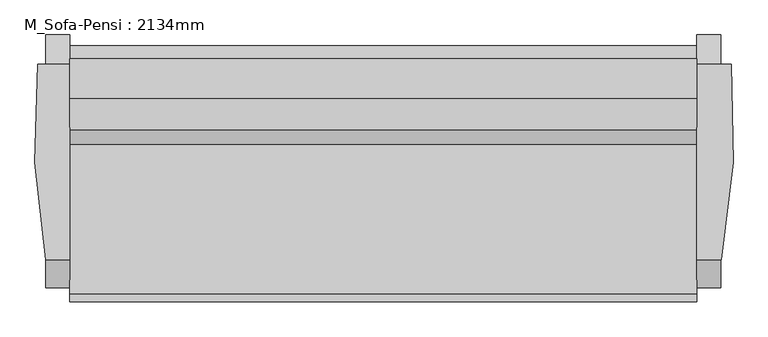
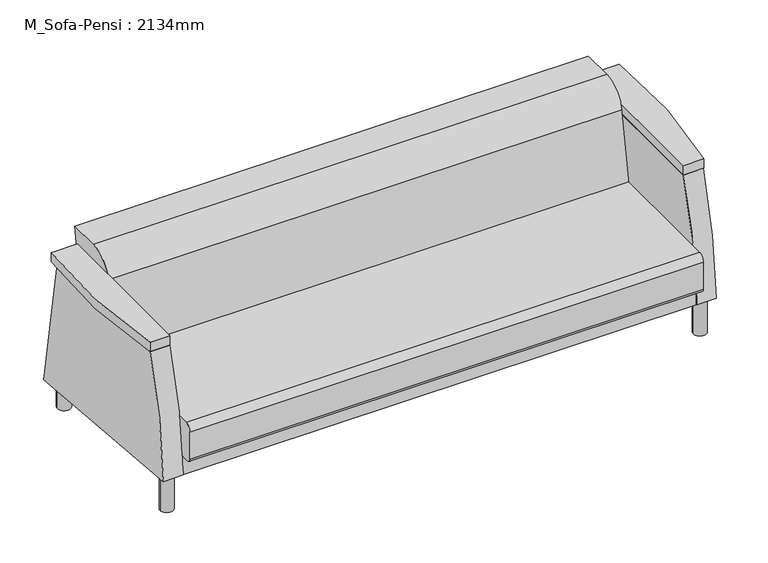
"""IFC4 building model written with IfcOpenShell, lengths in millimetres: furniture geometry, M_Sofa-Pensi : 2134mm."""

from ifc_helpers import new_model, si_unit, point, frame, frame_2d, origin, origin_with_axes, place, context, project, spatial, polyline, circle_curve, trimmed, segment, composite_curve, outline, extrude, source, transform, mapped, element, save
from ifc_brep_helpers import plane_surface, cylinder_surface, advanced_brep


def m_sofa_pensi_2134mm_91f3548c(model_context):
    return source(origin(), model_context, "Body", "SolidModel", [
        advanced_brep(
        [(1345.60625, 701.7619204, 79.3588346), (1345.60625, 608.6917937, 626.0203985), (1345.60625, -9.3943348, 626.0203985), (1345.60625, -97.7900405, 149.3105671), (1269.40625, -9.3943348, 626.0203985), (1269.40625, 608.6917937, 626.0203985), (1269.40625, 701.7619204, 79.3588346), (1269.40625, -83.3930704, 148.0509954), (1269.40625, 668.3047863, 148.0509954), (1269.40625, 668.3047863, 224.2509954), (1269.40625, -93.6952137, 224.2509954), (1269.40625, -93.6952137, 148.9523161), (1269.40625, -97.7900405, 149.3105671), (1269.40625, -93.6952137, 148.0509954), (-712.19375, -83.3930704, 148.0509954), (-712.19375, -93.6952137, 148.0509954), (-712.19375, -93.6952137, 148.9523161), (-712.19375, 668.3047863, 224.2509954), (-712.19375, -93.6952137, 224.2509954), (-712.19375, 668.3047863, 148.0509954), (-712.19375, 701.7619204, 79.3588346), (-712.19375, 608.6917937, 626.0203985), (-712.19375, -9.3943348, 626.0203985), (-712.19375, -97.7900405, 149.3105671), (-788.39375, -9.3943348, 626.0203985), (-788.39375, 608.6917937, 626.0203985), (-788.39375, 701.7619204, 79.3588346), (-788.39375, -97.7900405, 149.3105671)],
        [
            (0, 1),
            (1, 2),
            (2, 3, circle_curve(frame((1345.60625, 1499.9783711, 99.5888442), z_axis=(1.0, 0.0, 0.0), x_axis=(0.0, 1.0, 0.0)), 1598.5418814)),
            (3, 0),
            (4, 5),
            (5, 6),
            (6, 7),
            (7, 8),
            (8, 9),
            (9, 10),
            (10, 4, circle_curve(frame((1269.40625, 1499.9783711, 99.5888442), z_axis=(-1.0, 0.0, 0.0), x_axis=(0.0, 1.0, 0.0)), 1598.5418814)),
            (11, 12),
            (12, 10, circle_curve(frame((1269.40625, 1499.9783711, 99.5888442), z_axis=(-1.0, 0.0, 0.0), x_axis=(0.0, 1.0, 0.0)), 1598.5418814)),
            (10, 11),
            (0, 6),
            (5, 1),
            (4, 2),
            (12, 3),
            (11, 7),
            (11, 13),
            (13, 7),
            (14, 15),
            (15, 16),
            (16, 14),
            (9, 17),
            (17, 18),
            (18, 10),
            (18, 16),
            (15, 13),
            (14, 19),
            (19, 8),
            (19, 17),
            (20, 21),
            (21, 22),
            (22, 18, circle_curve(frame((-712.19375, 1499.9783711, 99.5888442), z_axis=(1.0, 0.0, 0.0), x_axis=(0.0, 1.0, 0.0)), 1598.5418814)),
            (14, 20),
            (18, 23, circle_curve(frame((-712.19375, 1499.9783711, 99.5888442), z_axis=(1.0, 0.0, 0.0), x_axis=(0.0, 1.0, 0.0)), 1598.5418814)),
            (23, 16),
            (24, 25),
            (25, 26),
            (26, 27),
            (27, 24, circle_curve(frame((-788.39375, 1499.9783711, 99.5888442), z_axis=(-1.0, 0.0, 0.0), x_axis=(0.0, 1.0, 0.0)), 1598.5418814)),
            (27, 23),
            (22, 24),
            (26, 20),
            (25, 21),
        ],
        [
            plane_surface(frame((1345.60625, 608.6917937, 626.0203985), z_axis=(1.0000000000000002, 0.0, 0.0), x_axis=(0.0, -0.16783676484789783, 0.985814800236531))),
            plane_surface(frame((1269.40625, 608.6917937, 626.0203985), z_axis=(-1.0000000000000002, 0.0, 0.0), x_axis=(0.0, 0.16783676484789783, -0.985814800236531))),
            plane_surface(frame((1345.60625, 701.7619204, 79.3588346), z_axis=(0.0, 0.985814800236531, 0.16783676484789783), x_axis=(-1.0, 0.0, 0.0))),
            plane_surface(frame((1345.60625, 608.6917937, 626.0203985), z_axis=(0.0, 0.0, 1.0), x_axis=(-1.0, 0.0, 0.0))),
            cylinder_surface(frame((1269.40625, 1499.9783711, 99.5888442), z_axis=(1.0, 0.0, 0.0), x_axis=(0.0, 1.0, 0.0)), 1598.5418814),
            plane_surface(frame((1345.60625, -97.7900405, 149.3105671), z_axis=(0.0, -0.08715574274767213, -0.9961946980917444), x_axis=(-1.0, 0.0, 0.0))),
            plane_surface(frame((1269.40625, -93.6952137, 224.2509954), z_axis=(1.0, 0.0, 0.0), x_axis=(0.0, -1.0, 0.0))),
            plane_surface(frame((-712.19375, -93.6952137, 224.2509954), z_axis=(-1.0, 0.0, 0.0), x_axis=(0.0, 1.0, 0.0))),
            plane_surface(frame((1269.40625, 668.3047863, 224.2509954), z_axis=(0.0, 0.0, 1.0), x_axis=(-1.0, 0.0, 0.0))),
            plane_surface(frame((1269.40625, -93.6952137, 224.2509954), z_axis=(0.0, -1.0, 0.0), x_axis=(-1.0, 0.0, 0.0))),
            plane_surface(frame((1269.40625, -93.6952137, 148.0509954), z_axis=(0.0, 0.0, -1.0), x_axis=(-1.0, 0.0, 0.0))),
            plane_surface(frame((1269.40625, 668.3047863, 148.0509954), z_axis=(0.0, 1.0, 0.0), x_axis=(-1.0, 0.0, 0.0))),
            plane_surface(frame((-712.19375, 3098.5202525, 99.5888442), z_axis=(1.0, 0.0, 0.0), x_axis=(0.0, 0.0, 1.0))),
            plane_surface(frame((-788.39375, 3098.5202525, 99.5888442), z_axis=(-1.0, 0.0, 0.0), x_axis=(0.0, 0.0, -1.0))),
            cylinder_surface(frame((-788.39375, 1499.9783711, 99.5888442), z_axis=(1.0, 0.0, 0.0), x_axis=(0.0, 1.0, 0.0)), 1598.5418814),
            plane_surface(frame((-712.19375, -97.7900405, 149.3105671), z_axis=(0.0, -0.08715574274766119, -0.9961946980917453), x_axis=(-1.0, 0.0, 0.0))),
            plane_surface(frame((-712.19375, 701.7619204, 79.3588346), z_axis=(0.0, 0.9858148002365317, 0.16783676484789375), x_axis=(-1.0, 0.0, 0.0))),
            plane_surface(frame((-712.19375, 608.6917937, 626.0203985), z_axis=(0.0, 0.0, 1.0), x_axis=(-1.0, 0.0, 0.0))),
        ],
        [
            (0, [[1, 2, 3, 4]]),
            (1, [[5, 6, 7, 8, 9, 10, 11]]),
            (1, [[12, 13, 14]]),
            (2, [[-1, 15, -6, 16]]),
            (3, [[-2, -16, -5, 17]]),
            (4, [[-3, -17, -11, -13, 18]]),
            (5, [[-4, -18, -12, 19, -7, -15]]),
            (6, [[20, 21, -19]]),
            (7, [[22, 23, 24]]),
            (8, [[25, 26, 27, -10]]),
            (9, [[-27, 28, -23, 29, -20, -14]]),
            (10, [[-29, -22, 30, 31, -8, -21]]),
            (11, [[-25, -9, -31, 32]]),
            (12, [[33, 34, 35, -26, -32, -30, 36]]),
            (12, [[37, 38, -28]]),
            (13, [[39, 40, 41, 42]]),
            (14, [[-42, 43, -37, -35, 44]]),
            (15, [[-41, 45, -36, -24, -38, -43]]),
            (16, [[-33, -45, -40, 46]]),
            (17, [[-34, -46, -39, -44]]),
        ],
    ),
        extrude(outline(composite_curve([segment(trimmed(circle_curve(frame_2d((-750.29375, -53.0901639)), 25.4), [point((-775.69375, -53.0901639))], [point((-724.89375, -53.0901639))], False, "CARTESIAN"), True, "CONTINUOUS"), segment(trimmed(circle_curve(frame_2d((-750.29375, -53.0901639)), 25.4), [point((-724.89375, -53.0901639))], [point((-775.69375, -53.0901639))], False, "CARTESIAN"), True, "CONTINUOUS")], self_intersect=False)), origin_with_axes(), (0.0, 0.0, 1.0), 148.43125),
        extrude(outline(composite_curve([segment(trimmed(circle_curve(frame_2d((-750.29375, 632.7098361)), 25.4), [point((-775.69375, 632.7098361))], [point((-724.89375, 632.7098361))], False, "CARTESIAN"), True, "CONTINUOUS"), segment(trimmed(circle_curve(frame_2d((-750.29375, 632.7098361)), 25.4), [point((-724.89375, 632.7098361))], [point((-775.69375, 632.7098361))], False, "CARTESIAN"), True, "CONTINUOUS")], self_intersect=False)), origin_with_axes(), (0.0, 0.0, 1.0), 148.43125),
        extrude(outline(composite_curve([segment(trimmed(circle_curve(frame_2d((1307.50625, 632.7098361)), 25.4), [point((1282.10625, 632.7098361))], [point((1332.90625, 632.7098361))], False, "CARTESIAN"), True, "CONTINUOUS"), segment(trimmed(circle_curve(frame_2d((1307.50625, 632.7098361)), 25.4), [point((1332.90625, 632.7098361))], [point((1282.10625, 632.7098361))], False, "CARTESIAN"), True, "CONTINUOUS")], self_intersect=False)), origin_with_axes(), (0.0, 0.0, 1.0), 148.43125),
        extrude(outline(composite_curve([segment(trimmed(circle_curve(frame_2d((1307.50625, -53.0901639)), 25.4), [point((1282.10625, -53.0901639))], [point((1332.90625, -53.0901639))], False, "CARTESIAN"), True, "CONTINUOUS"), segment(trimmed(circle_curve(frame_2d((1307.50625, -53.0901639)), 25.4), [point((1332.90625, -53.0901639))], [point((1282.10625, -53.0901639))], False, "CARTESIAN"), True, "CONTINUOUS")], self_intersect=False)), origin_with_axes(), (0.0, 0.0, 1.0), 148.43125),
        extrude(outline(composite_curve([segment(trimmed(circle_curve(frame_2d((-116.5901639, 351.2509954)), 25.4), [point((-141.9901639, 351.2509954))], [point((-116.5901639, 376.6509954))], False, "CARTESIAN"), True, "CONTINUOUS"), segment(polyline([(-116.5901639, 376.6509954), (355.3895541, 376.6509954), (402.1988177, 642.1195211)]), True, "CONTINUOUS"), segment(trimmed(circle_curve(frame_2d((502.2552854, 624.4768662)), 101.6), [point((402.1988177, 642.1195211))], [point((502.2552854, 726.0768662))], False, "CARTESIAN"), True, "CONTINUOUS"), segment(polyline([(502.2552854, 726.0768662), (626.3344485, 726.0768662), (609.5377828, 620.1719187), (667.6541767, 224.2509954), (-126.1151639, 224.2509954)]), True, "CONTINUOUS"), segment(trimmed(circle_curve(frame_2d((-126.1151639, 240.1259954)), 15.875), [point((-126.1151639, 224.2509954))], [point((-141.9901639, 240.1259954))], False, "CARTESIAN"), True, "CONTINUOUS"), segment(polyline([(-141.9901639, 240.1259954), (-141.9901639, 351.2509954)]), True, "CONTINUOUS")], self_intersect=False)), frame((-712.19375, 0.0, 0.0), z_axis=(1.0, 0.0, 0.0), x_axis=(0.0, 1.0, 0.0)), (0.0, 0.0, 1.0), 1981.6),
        extrude(outline(composite_curve([segment(polyline([(-712.19375, -9.3943348), (-788.39375, -9.3943348)]), True, "CONTINUOUS"), segment(trimmed(circle_curve(frame_2d((1379.7527561, 389.2697363)), 2204.4936638), [point((-788.39375, -9.3943348))], [point((-813.79375, 608.6917935))], False, "CARTESIAN"), True, "CONTINUOUS"), segment(polyline([(-813.79375, 608.6917935), (-712.19375, 608.6917935), (-712.19375, -9.3943348)]), True, "CONTINUOUS")], self_intersect=False)), frame((0.0, 0.0, 626.0203985), z_axis=(0.0, 0.0, 1.0), x_axis=(1.0, 0.0, 0.0)), (0.0, 0.0, 1.0), 38.1),
        extrude(outline(composite_curve([segment(polyline([(1269.40625, -9.3943348), (1269.40625, 608.9395268), (1378.0864453, 608.9395268)]), True, "CONTINUOUS"), segment(trimmed(circle_curve(frame_2d((-821.5771494, 407.0270204)), 2208.9111775), [point((1378.0864453, 608.9395268))], [point((1347.7273117, -9.3943348))], False, "CARTESIAN"), True, "CONTINUOUS"), segment(polyline([(1347.7273117, -9.3943348), (1269.40625, -9.3943348)]), True, "CONTINUOUS")], self_intersect=False)), frame((0.0, 0.0, 626.0203985), z_axis=(0.0, 0.0, 1.0), x_axis=(1.0, 0.0, 0.0)), (0.0, 0.0, 1.0), 38.1),
    ])


if __name__ == "__main__":
    model = new_model("IFC4")
    model_context = context("Model", 3, world=origin())
    ifc_project = project(units=[si_unit("LENGTHUNIT", "METRE", prefix="MILLI")], contexts=[model_context])
    site = spatial("IfcSite", under=ifc_project)
    building = spatial("IfcBuilding", under=site)
    placement = place(None, origin())
    m_sofa_pensi_2134mm_shape = m_sofa_pensi_2134mm_91f3548c(model_context)
    element("IfcFurniture", 1, ObjectType="M_Sofa-Pensi : 2134mm", at=placement, inside=building, context=model_context, shape_type="MappedRepresentation", body=[
        mapped(m_sofa_pensi_2134mm_shape, transform((0.0, 0.0, 0.0), x_axis=(1.0, 0.0, 0.0), y_axis=(0.0, 1.0, 0.0), z_axis=(0.0, 0.0, 1.0))),
    ])
    save(model, "model.ifc")

# Revit data of these elements
# Type "M_Sofa-Pensi : 2134mm"
#   Length = 2134 mm
#   Sofa Material = Linen, Beige
#   Frame Material = Steel, Chrome Plated
#   Default Elevation = 0
# Element 1 (IfcFurniture, "M_Sofa-Pensi : 2134mm")
#   Materials on its faces: "Linen, Beige", "Steel, Chrome Plated"
# Materials
#   "Linen, Beige": class "Textile", colour RGB 249 239 230, transparency 0, Description = "Linen, beige", Cost = 0
#   "Steel, Chrome Plated": class "Metal", colour RGB 244 244 244, transparency 0, Description = "Chromiuim plated steel", Cost = 0
